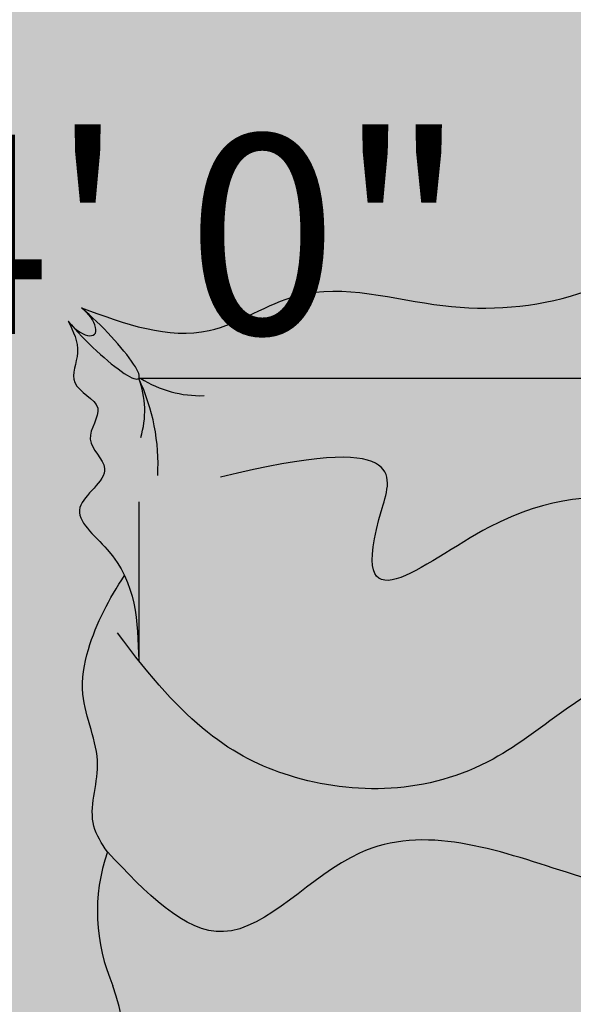
# Model space of a CAD drawing. Units: inches. Extents: x 1704 to 6393, y -157 to 1172.
# Tile 36 of 122: x 2488 to 2526, y 148 to 215. Entities that reach past the tile are written whole.
import ezdxf

# ---------------------------------------------------------------- set-up
doc = ezdxf.new("R2010")
doc.units = ezdxf.units.IN
doc.header["$MEASUREMENT"] = 0
for name, color, linetype, lineweight in [('A-ANNO-DIMS', 7, 'Continuous', 13), ('A-FURN', 8, 'Continuous', 18), ('estofado', 7, 'Continuous', 25)]:
    doc.layers.add(name, color=color, linetype=linetype, lineweight=lineweight)
doc.layers.add('A-FLOR-PATT', color=7, linetype='Continuous', lineweight=13, true_color=0xf2f2f2)
doc.styles.get("Standard").update_dxf_attribs({"font": 'arial.ttf'})
doc.dimstyles.get("Standard").update_dxf_attribs({"dimtxt": 6, "dimasz": 2, "dimexe": 0.18, "dimexo": 0.0625, "dimgap": 0.09, "dimtad": 0, "dimtih": 1, "dimtoh": 1, "dimdec": 1, "dimzin": 0, "dimdsep": 46, "dimlunit": 3, "dimtxsty": 'Standard', "dimblk": 'ARCHTICK', "dimcen": 0.09, "dimadec": 0, "dimazin": 0, "dimtfac": 1, "dimtdec": 1, "dimtofl": 0, "dimtmove": 0, "dimatfit": 3, "dimfxl": 1, "dimtolj": 1, "dimtzin": 0, "dimarcsym": 0})

# ---------------------------------------------------------------- blocks, each defined once
blk = doc.blocks.new('Cama Box Regencia LOLA')
at = {"layer": 'estofado', "ltscale": 0.2}
h = blk.add_hatch(color=256, dxfattribs=at)
h.dxf.hatch_style = 1
h.set_gradient(color1=(240, 232, 219), color2=(213, 190, 154), one_color=1, tint=0.7200000286102295, name='CURVED')
edge = h.paths.add_edge_path()
edge.add_spline(control_points=[(0.343533776195045, -0.8455058148597345), (0.2879313990920309, -0.8167160606696484), (0.2054770794474052, -0.7744470032542381), (0.0954193394759386, -0.7742416952675626), (-0.0885363502328574, -0.7276964167006668), (0.2428192566063672, -0.7672518992321216), (0.345087521536243, -0.8076697826234067), (0.3825206986321063, -0.8228555492498799)], knot_values=[0.0056315103357428, 0.0056315103357428, 0.0056315103357428, 0.0056315103357428, 0.1860138916206105, 0.2660015162584448, 0.3570871810327863, 0.5963901805690979, 0.739731738908988, 0.739731738908988, 0.739731738908988, 0.739731738908988], degree=3, periodic=0)
edge.add_spline(control_points=[(0.3825206986325611, -0.8228555492497662), (0.3974221570828149, -0.8135511441712424), (0.4121061736600496, -0.8037181558521524), (0.4266849906532571, -0.7937075488799225)], knot_values=[1.358237767273279, 1.358237767273279, 1.358237767273279, 1.358237767273279, 1.409915662372559, 1.409915662372559, 1.409915662372559, 1.409915662372559], degree=3, periodic=0)
edge.add_spline(control_points=[(0.4266849905698109, -0.7937075489369932), (0.3998777739682282, -0.7821381809783361), (0.3476761897024971, -0.7634757898491671), (0.2670618099601825, -0.7565375622627358), (0.0835725072796549, -0.7192994417154637), (0.288524529784695, -0.7446405493717521), (0.4247448861246994, -0.7759943071475277), (0.4449816270193879, -0.7810438091316882)], knot_values=[0.1043639306803623, 0.1043639306803623, 0.1043639306803623, 0.1043639306803623, 0.1896363068641149, 0.2696239315019491, 0.3607095962762907, 0.6000125958126024, 0.6446217338078729, 0.6446217338078729, 0.6446217338078729, 0.6446217338078729], degree=3, periodic=0)
edge.add_spline(control_points=[(0.4449816270197289, -0.7810438091316882), (0.5029779388527232, -0.7406836481117695), (0.5966687145296419, -0.6736247633211292), (0.7071737530245628, -0.6656573253703187), (0.7517012483331201, -0.6672238302253392)], knot_values=[1.43159032281798, 1.43159032281798, 1.43159032281798, 1.43159032281798, 1.63814180148235, 1.770695287284994, 1.770695287284994, 1.770695287284994, 1.770695287284994], degree=3, periodic=0)
edge.add_arc((0.7481853615017826, -0.767162003811734), 0.0999999999999888, 58.7920033978138, 87.98512997550938, ccw=False)
edge.add_line((0.8000000000000682, -0.6816328085782289), (0.8000000000000682, -0.154802362840428))
edge.add_line((0.8000000000000682, -0.154802362840428), (-0.7999999999999546, -0.154802362840428))
edge.add_line((-0.7999999999999546, -0.154802362840428), (-0.8000000000000682, -0.7409839258539819))
edge.add_spline(control_points=[(-0.799999999999841, -0.7409839258539251), (-0.7846451382113174, -0.74846387981205), (-0.7568940913494089, -0.7651582159765554), (-0.7559936909002545, -0.8096905380045313), (-0.7049413305308008, -0.8142555457367848), (-0.7013836936888538, -0.8139988647640733)], knot_values=[0.0122267587020837, 0.0122267587020837, 0.0122267587020837, 0.0122267587020837, 0.0594720782072034, 0.1062176618094138, 0.134458043575382, 0.134458043575382, 0.134458043575382, 0.134458043575382], degree=3, periodic=0)
edge.add_spline(control_points=[(-0.7013836936890812, -0.8139988647637892), (-0.6428309483887916, -0.8132695376718857), (-0.532520673001045, -0.8118955240036598), (-0.2390712668254764, -0.6717984706609172), (-0.3892411364554391, -0.7557901092520752), (-0.4591093260188473, -0.8070101468627512), (-0.5571511178645779, -0.795652750469742), (-0.608497950975675, -0.8409486634728295), (-0.6632498050151981, -0.8266781836207997), (-0.6991149398675134, -0.8254126024436914), (-0.719552182989446, -0.8246914287938125)], knot_values=[0, 0, 0, 0, 0.2187005959148062, 0.4120203559900679, 0.4786136596093368, 0.6046444033330721, 0.6969970394608519, 0.7456449795902803, 0.7925683322559657, 0.8547274388453192, 0.8547274388453192, 0.8547274388453192, 0.8547274388453192], degree=3, periodic=0)
edge.add_spline(control_points=[(-0.7195521829781911, -0.824691428792164), (-0.7293124663336812, -0.8248308281530967), (-0.7545977292818407, -0.8216412233076653), (-0.7742556984202338, -0.794819860189591), (-0.7939222919129634, -0.7820064600295497), (-0.799999999999841, -0.7800193173443404)], knot_values=[0.1564883932805935, 0.1564883932805935, 0.1564883932805935, 0.1564883932805935, 0.184397548386913, 0.2313764834161266, 0.2505984550882281, 0.2505984550882281, 0.2505984550882281, 0.2505984550882281], degree=3, periodic=0)
edge.add_line((-0.8000000000000682, -0.7800193173444541), (-0.7999999999999546, -0.8218505664627286))
edge.add_spline(control_points=[(-0.7999999999999546, -0.8218505664625013), (-0.7938082505512511, -0.8290217081292894), (-0.7673857405620766, -0.8512914803976059), (-0.7619109683460011, -0.8661369353891359), (-0.6555700939965164, -0.8510070218793543), (-0.7139793977868294, -0.8637526923380391), (-0.7379026254519659, -0.8623504601624176), (-0.7688129786438367, -0.8813042143888196), (-0.7854260296310259, -0.8561610219318254), (-0.7961930533253962, -0.8566031243811949), (-0.7999999999999546, -0.8573491405791173)], knot_values=[0.0595743221876141, 0.0595743221876141, 0.0595743221876141, 0.0595743221876141, 0.08075289116965, 0.1037414994169835, 0.1697200936249022, 0.1760361327243865, 0.2071371586311508, 0.2404744334261798, 0.2623408547027293, 0.2736604507987723, 0.2736604507987723, 0.2736604507987723, 0.2736604507987723], degree=3, periodic=0)
edge.add_line((-0.7999999999999546, -0.8573491405791173), (-0.8000000000000682, -0.9113562424721521))
edge.add_spline(control_points=[(-0.8000000000000682, -0.9113562424720385), (-0.7937204054647964, -0.9077594990848183), (-0.7710343135782978, -0.8978798065321029), (-0.7213062468074442, -0.9144666877443228), (-0.6268586829058905, -0.862430497409548), (-0.6896594748232019, -0.9045634991654196), (-0.7483442493064559, -0.9189273406958591), (-0.7835301183422417, -0.922920432793262), (-0.7896301351460125, -0.9477657000142585), (-0.7975786973822779, -0.955260590410262), (-0.8000000000001818, -0.9571831923294098)], knot_values=[0.0138560263374175, 0.0138560263374175, 0.0138560263374175, 0.0138560263374175, 0.0348737775836104, 0.0888666909546002, 0.1078792274429341, 0.1267378491223226, 0.1587140219647659, 0.1937574699451985, 0.2174867851300671, 0.2267221218327879, 0.2267221218327879, 0.2267221218327879, 0.2267221218327879], degree=3, periodic=0)
edge.add_line((-0.7999999999999546, -0.957183192329296), (-0.7999999999999546, -1.145824641594742))
edge.add_spline(control_points=[(-0.8000000000002955, -1.145824641594913), (-0.7271039467997298, -1.094596787649038), (-0.4885706936571524, -0.9465888221489535), (-0.0701640902225336, -0.9707493165000187), (0.237911901821235, -0.902164522332157), (0.3435337762145991, -0.845505814843193)], knot_values=[0.1168958193629841, 0.1168958193629841, 0.1168958193629841, 0.1168958193629841, 0.3797203297758731, 0.9577018633805092, 1.31379338443587, 1.31379338443587, 1.31379338443587, 1.31379338443587], degree=3, periodic=0)
h.paths.add_polyline_path([(-0.6766340706021765, -0.6101327540145576, -0.3575266660906883), (-0.7312746368313583, -0.6354535276154252, -0.3575266660894137), (-0.7059538632299791, -0.5808129613865844, -0.1647847126465284), (-0.7059538632300928, -0.2676124402649407, -0.3575266660890756), (-0.7312746368312446, -0.2129718740360431, -0.3575266660908716), (-0.6766340706020629, -0.2382926476369676, -0.0925607043966334), (-0.1295169377724505, -0.2382926476369107, -0.3575266660898965), (-0.0748763715433825, -0.2129718740360431, -0.3575266660894428), (-0.1001971451446479, -0.2676124402649407, -0.1647847126465285), (-0.1001971451445343, -0.5808129613865844, -0.3575266660890756), (-0.0748763715433825, -0.6354535276154821, -0.3575266660898962), (-0.1295169377724505, -0.6101327540146145, -0.0925607043966531)], flags=16)
h.paths.add_polyline_path([(0.0748763715433825, -0.6354535276157094, -0.3575266660910266), (0.1001971451446479, -0.5808129613865844, -0.1647847126465284), (0.1001971451445343, -0.2676124402649407, -0.3575266660890757), (0.0748763715433825, -0.2129718740360431, -0.3575266660898962), (0.1295169377724505, -0.2382926476369107, -0.0925607043966334), (0.6766340706020629, -0.2382926476369676, -0.3575266660908718), (0.7312746368312446, -0.2129718740360431, -0.3575266660894425), (0.7059538632299791, -0.2676124402649407, -0.1647847126465283), (0.7059538632300928, -0.5808129613865844, -0.3575266660890756), (0.7312746368312446, -0.6354535276154821, -0.3575266660908716), (0.6766340706020629, -0.6101327540145576, -0.0925607043966335), (0.1295169377724505, -0.6101327540146145, -0.3575266660906303)], flags=16)
h = blk.add_hatch(color=256, dxfattribs=at)
h.dxf.hatch_style = 1
h.set_gradient(color1=(206, 178, 131), color2=(227, 212, 186), one_color=1, tint=0.8100000023841857, name='CYLINDER')
edge = h.paths.add_edge_path()
edge.add_arc((0.7481853614966667, -0.7671620038115634), 0.0999999999999888, 342.0511336145294, 447.9851299725766)
edge.add_spline(control_points=[(0.7517012483331201, -0.6672238302253392), (0.7071737530245628, -0.6656573253703187), (0.5966687145298692, -0.6736247633211292), (0.5029779388527232, -0.7406836481117125), (0.4449816270195015, -0.7810438091316314)], knot_values=[1.431590322817835, 1.431590322817835, 1.431590322817835, 1.431590322817835, 1.564143808620479, 1.770695287284994, 1.770695287284994, 1.770695287284994, 1.770695287284994], degree=3, periodic=0)
edge.add_spline(control_points=[(0.4449816270195015, -0.7810438091316314), (0.4388957332065502, -0.7852790380018178), (0.4327996148541616, -0.7895089160493285), (0.4266849906533708, -0.7937075488798087)], knot_values=[1.409915662372814, 1.409915662372814, 1.409915662372814, 1.409915662372814, 1.431590322817835, 1.431590322817835, 1.431590322817835, 1.431590322817835], degree=3, periodic=0)
edge.add_spline(control_points=[(0.4266849906533708, -0.7937075488798087), (0.4121061736600496, -0.8037181558521524), (0.3974221570825875, -0.8135511441712991), (0.38252069863222, -0.8228555492498799)], knot_values=[1.358237767273037, 1.358237767273037, 1.358237767273037, 1.358237767273037, 1.409915662372815, 1.409915662372815, 1.409915662372815, 1.409915662372815], degree=3, periodic=0)
edge.add_line((0.3825206986330158, -0.8228555492493114), (0.343533776286904, -0.8455058148063584))
edge.add_spline(control_points=[(0.3435337761924302, -0.8455058148550165), (0.2379119018048641, -0.902164522335795), (-0.0701640902311738, -0.9707493164995071), (-0.4885706936571524, -0.9465888221488967), (-0.7271039467997298, -1.094596787649038), (-0.8000000000000682, -1.145824641594742)], knot_values=[0.1168958193630798, 0.1168958193630798, 0.1168958193630798, 0.1168958193630798, 0.472987340393773, 1.050968873998409, 1.313793384411202, 1.313793384411202, 1.313793384411202, 1.313793384411202], degree=3, periodic=0)
edge.add_spline(control_points=[(-0.8000000000000682, -1.145824641594742), (-0.8038896190357718, -1.14855807951244), (-0.8077744942224853, -1.151305646504738), (-0.8116551946761774, -1.154065647517199)], knot_values=[0.1028719158199011, 0.1028719158199011, 0.1028719158199011, 0.1028719158199011, 0.1168958193630799, 0.1168958193630799, 0.1168958193630799, 0.1168958193630799], degree=3, periodic=0)
edge.add_arc((-0.7536973518524519, -1.235557294053705), 0.1000000000000352, 125.4208969883762, 169.6981795679068)
edge.add_spline(control_points=[(-0.852085287466366, -1.217673946333093), (-0.8521399740518518, -1.217974812833915), (-0.8565649010855622, -1.242328483616745), (-0.8662697220019026, -1.297321141147904), (-0.8487158298532904, -1.34896742172242), (-0.8348745804664758, -1.381844109035796)], knot_values=[0.3128349436863077, 0.3128349436863077, 0.3128349436863077, 0.3128349436863077, 0.3137509534211996, 0.386958004641742, 0.4759027329026081, 0.4759027329026081, 0.4759027329026081, 0.4759027329026081], degree=3, periodic=0)
edge.add_spline(control_points=[(-0.8348745804664758, -1.38184410903591), (-0.8226532004149476, -1.367823298399059), (-0.8056354908857201, -1.352141651537124), (-0.7460155199962628, -1.32170802000337)], knot_values=[0.0062456970656236, 0.0062456970656236, 0.0062456970656236, 0.0062456970656236, 0.0554759259147193, 0.0554759259147193, 0.0554759259147193, 0.0554759259147193], degree=3, periodic=0)
edge.add_spline(control_points=[(-0.7460155200169539, -1.321708019985464), (-0.6188339616464873, -1.25080943574278), (-0.3488365122128698, -1.179158668568902), (0.0338148848931041, -1.279726484458706), (0.3977250465933366, -1.412092721352792), (0.6449024721503065, -1.106270719748692), (0.7873766543807506, -1.256744909425322), (0.8547271521993025, -1.327877176513538)], knot_values=[0.0991852523588446, 0.0991852523588446, 0.0991852523588446, 0.0991852523588446, 0.5236467270390676, 0.9270872950244264, 1.289918234564769, 1.564439021262726, 1.810554634340498, 1.810554634340498, 1.810554634340498, 1.810554634340498], degree=3, periodic=0)
edge.add_arc((0.5509678495186563, -1.223443291813453), 0.3212104454069235, 341.0267878798241, 383.7782184284114)
edge.add_arc((1.292676354991499, -0.9435407756057543), 0.4723459732861395, 162.0511336103901, 198.5657216587827, ccw=False)
h = blk.add_hatch(color=256, dxfattribs=at)
h.dxf.hatch_style = 1
h.set_gradient(color1=(206, 178, 131), color2=(233, 221, 200), one_color=1, tint=0.8500000238418579, name='CURVED')
edge = h.paths.add_edge_path()
edge.add_spline(control_points=[(0.9233883396182136, -2.254908822900802), (0.9143712174658276, -2.237158585978875), (0.8971704820246486, -2.20329887728792), (0.9295105801843419, -2.140290914518345), (0.848651568119294, -2.10957861148239), (0.9047062348403186, -2.046222426005954), (0.8299480774321636, -1.990932361540615), (0.9387479200587449, -1.92692496801726), (0.8590435458045249, -1.86767849203585), (0.8322262745575699, -1.826028043643361), (0.8247981799574972, -1.810442049687992)], knot_values=[0, 0, 0, 0, 0.0575832900035364, 0.1098437972159638, 0.1698138218664432, 0.2255174829302509, 0.2824861515521905, 0.3632291183773252, 0.4509842065695901, 0.5012091817853866, 0.5012091817853866, 0.5012091817853866, 0.5012091817853866], degree=3, periodic=0)
edge.add_spline(control_points=[(0.8247981799572698, -1.810442049688447), (0.8512430237993839, -1.769990096378137), (0.8869160776755506, -1.705010622333873), (0.9070359522544322, -1.586338752195842), (0.8536462472426364, -1.488247672851343), (0.8944567470317679, -1.387739666353695), (0.8643796102055603, -1.342420998864781), (0.8547271521993025, -1.327877176513538)], knot_values=[0, 0, 0, 0, 0.1438744691785906, 0.2224893870322766, 0.3492927143212738, 0.4561786976395368, 0.5066917301592304, 0.5066917301592304, 0.5066917301592304, 0.5066917301592304], degree=3, periodic=0)
edge.add_spline(control_points=[(0.8547271521993025, -1.327877176513538), (0.7873766543807506, -1.256744909425322), (0.6449024721503065, -1.106270719748692), (0.3977250465933366, -1.412092721352792), (0.0338148848931041, -1.279726484458706), (-0.3488365122128698, -1.179158668568902), (-0.6188339616464873, -1.25080943574278), (-0.7460155200169539, -1.321708019985464)], knot_values=[0.0991852523588446, 0.0991852523588446, 0.0991852523588446, 0.0991852523588446, 0.3453008654366167, 0.6198216521345741, 0.9826525916749167, 1.386093159660275, 1.810554634340498, 1.810554634340498, 1.810554634340498, 1.810554634340498], degree=3, periodic=0)
edge.add_spline(control_points=[(-0.7460155199962628, -1.32170802000337), (-0.8056354908857201, -1.352141651537124), (-0.8226532004149476, -1.367823298399059), (-0.8348745804664758, -1.38184410903591)], knot_values=[0.0062456970656236, 0.0062456970656236, 0.0062456970656236, 0.0062456970656236, 0.0554759259147193, 0.0554759259147193, 0.0554759259147193, 0.0554759259147193], degree=3, periodic=0)
edge.add_spline(control_points=[(-0.8348745804664758, -1.38184410903591), (-0.8364250716851984, -1.383622888820184), (-0.8378983647115774, -1.385374937005849), (-0.8393716577378427, -1.387126985191514)], knot_values=[0, 0, 0, 0, 0.0062456970656236, 0.0062456970656236, 0.0062456970656236, 0.0062456970656236], degree=3, periodic=0)
edge.add_arc((-0.6180450437709624, -1.576392779500167), 0.2912164331649039, 139.4648411061637, 203.3711573294546)
edge.add_arc((-0.7011750866292914, -1.609837078845487), 0.2016528082906132, 204.0179006417974, 212.6189639884946)
edge.add_spline(control_points=[(-0.8710220093900034, -1.718537943240505), (-0.8696870122217887, -1.721658691442996), (-0.8597709916446092, -1.746046247230935), (-0.8464685798230674, -1.804421032451443), (-0.888988689927828, -1.889951451602371), (-0.8378676506146121, -1.973422824210047), (-0.8371590179440318, -2.05992368952792), (-0.8871569320951948, -2.144598622072578), (-0.908935644436724, -2.210906123939594), (-0.9233883398977695, -2.254908823284267)], knot_values=[0, 0, 0, 0, 0.0101500649009363, 0.0785829584511912, 0.1732273504791735, 0.2688802694005398, 0.3498050162211252, 0.4202002266429896, 0.5590752189863636, 0.5590752189863636, 0.5590752189863636, 0.5590752189863636], degree=3, periodic=0)
edge.add_ellipse((-0.9040800600764669, -2.258882422916315), major_axis=(0.0267880171833212, 0.0267880171833213), ratio=0.4535320972039226, start_angle=94.15910660291303, end_angle=123.37101895145429, ccw=False)
edge.add_ellipse((-0.8772920428931456, -2.232094405732993), major_axis=(0.0772920428927364, 0.0772920428927364), ratio=0.168252450050839, start_angle=-1.0527401173021644e-10, end_angle=156.3071135567154, ccw=False)
edge.add_line((-0.8000000000002955, -2.154802362840428), (0.7999592378284888, -2.154802362840428))
edge.add_arc((0.9462065466516378, -2.098298447668867), 0.1567831871334379, 200.9447658774159, 201.1244713640487, ccw=False)
edge.add_arc((1.115979327553759, -2.004946707326951), 0.3497136727815615, 205.2898146244752, 205.3730108333857)
edge.add_ellipse((0.8772920428930319, -2.232094405732993), major_axis=(-0.0772920428927364, 0.0772920428927364), ratio=0.168252450050839, start_angle=203.6928864432847, end_angle=359.99999999994674, ccw=False)
edge.add_ellipse((0.9040800600763532, -2.258882422916315), major_axis=(-0.0267880171833213, 0.0267880171833213), ratio=0.4535320972039226, start_angle=236.6289810485458, end_angle=265.84089339708703, ccw=False)
h = blk.add_hatch(color=256, dxfattribs=at)
h.dxf.hatch_style = 1
h.set_gradient(color1=(206, 178, 131), color2=(233, 221, 200), one_color=1, tint=0.8500000238418579, name='CURVED')
edge = h.paths.add_edge_path()
edge.add_spline(control_points=[(-0.9001064604443627, -2.27819070273756), (-0.866259371332262, -2.263084355976445), (-0.8028331991894219, -2.234776522858453), (-0.7685206103102474, -2.343981002846874), (-0.6122536186376238, -2.322828464485212), (-0.4353754265674752, -2.183795504726106), (-0.2043351766035357, -2.412166101990749), (0.035742157155596, -2.28434544697319), (0.2724023732024534, -2.265741378418681), (0.4990197572961961, -2.339647395113615), (0.6925408411253784, -2.202138696866825), (0.8240737498149427, -2.250332331133733), (0.900106460444249, -2.27819070273756)], knot_values=[0, 0, 0, 0, 0.0915194039844232, 0.1714985135733706, 0.2551966802733756, 0.4993431682155844, 0.7776132872898075, 0.9991109890269537, 1.23769004728933, 1.492615491211055, 1.658192352121012, 1.885025012049534, 1.885025012049534, 1.885025012049534, 1.885025012049534], degree=3, periodic=0)
edge.add_ellipse((0.9040800600763532, -2.258882422916315), major_axis=(-0.0267880171833213, 0.0267880171833213), ratio=0.4535320972039226, start_angle=454.1591066084853, end_angle=483.3710189511271, ccw=False)
edge.add_ellipse((0.8772920428930319, -2.232094405732993), major_axis=(-0.0772920428927364, 0.0772920428927364), ratio=0.168252450050839, start_angle=359.99999999994674, end_angle=516.3071135577263, ccw=False)
edge.add_arc((0.9462065466977946, -2.098298447788181), 0.1567831871334379, 201.1244713173118, 201.142614633458, ccw=False)
edge.add_line((0.7999592378286025, -2.154802362840428), (-0.8000000000004092, -2.154802362840428))
edge.add_ellipse((-0.8772920428931456, -2.232094405732993), major_axis=(0.0772920428927364, 0.0772920428927364), ratio=0.168252450050839, start_angle=-156.3071135577261, end_angle=-1.0527401173021644e-10, ccw=False)
edge.add_ellipse((-0.9040800600764669, -2.258882422916315), major_axis=(0.0267880171833212, 0.0267880171833213), ratio=0.4535320972039226, start_angle=-123.3710189511271, end_angle=-94.15910660848522, ccw=False)
h = blk.add_hatch(color=256, dxfattribs=at)
h.dxf.hatch_style = 1
h.set_gradient(color1=(206, 178, 131), color2=(233, 221, 200), one_color=1, tint=0.8500000238418579, name='CURVED')
edge = h.paths.add_edge_path()
edge.add_ellipse((0.8772920428930319, -2.232094405732993), major_axis=(-0.0772920428927364, 0.0772920428927364), ratio=0.168252450050839, start_angle=203.6928864432846, end_angle=359.9999999999468)
edge.add_ellipse((0.8772920428930319, -2.232094405732993), major_axis=(-0.0772920428927364, 0.0772920428927364), ratio=0.168252450050839, start_angle=359.9999999999468, end_angle=516.3071135577261)
edge.add_ellipse((0.9040800600763532, -2.258882422916315), major_axis=(-0.0267880171833213, 0.0267880171833213), ratio=0.4535320972039226, start_angle=265.84089339708703, end_angle=454.1591066084853, ccw=False)
for p, q in [((0.8000000000000682, -1.939064283336335), (0.8000000000000682, -1.662039728679133)), ((-0.7999999999999546, -2.154802362840428), (0.8000000000000682, -2.154802362840428))]:
    blk.add_line(p, q, dxfattribs=at)
for centre, radius, start, end in [((1.292676354991613, -0.9435407756055268), 0.4723459732861117, 162.0511336104213, 198.5657216589983), ((0.55096784951877, -1.223443291813453), 0.3212104454069235, 341.0267878798186, 23.77821842812888), ((1.115979327644367, -2.00494670751874), 0.3497136727815545, 176.7524727679717, 205.3730107986517), ((0.9462065466502735, -2.098298447665399), 0.1567831871334492, 162.6474673821321, 201.1361021892849), ((0.6916068347399005, -2.322769188842187), 0.1980600766927276, 58.0012856468178, 91.6550645032879)]:
    blk.add_arc(centre, radius, start, end, dxfattribs=at)
for centre, major_axis, ratio, start_param, end_param in [((0.8772920428930319, -2.232094405732993), (-0.0772920428927364, 0.0772920428927364), 0.168252450050839, 4.250341947992563, 8.31602866635556), ((0.9040800600763532, -2.258882422916315), (-0.0267880171833213, 0.0267880171833213), 0.4535320972039226, 4.422106649467695, 8.144263964888069)]:
    blk.add_ellipse(centre, major_axis=major_axis, ratio=ratio, start_param=start_param, end_param=end_param, dxfattribs=at)
for points, knots in [([(-0.8116551946761774, -1.154065647517199), (-0.7350455857787211, -1.099579968801037), (-0.493473113061782, -0.9463057365681493), (-0.0701640902311738, -0.9707493164995071), (0.2379119018048641, -0.902164522335795), (0.3435337761924302, -0.8455058148550165)], [0.1028719158199011, 0.1028719158199011, 0.1028719158199011, 0.1028719158199011, 0.3797203297758731, 0.9577018633805092, 1.313793384411202, 1.313793384411202, 1.313793384411202, 1.313793384411202]), ([(-0.7460155200169539, -1.321708019985464), (-0.6188339616464873, -1.25080943574278), (-0.3488365122128698, -1.179158668568902), (0.0338148848931041, -1.279726484458706), (0.3977250465933366, -1.412092721352792), (0.6449024721503065, -1.106270719748692), (0.7873766543807506, -1.256744909425322), (0.8547271521993025, -1.327877176513538)], [0.0991852523588446, 0.0991852523588446, 0.0991852523588446, 0.0991852523588446, 0.5236467270390676, 0.9270872950244264, 1.289918234564769, 1.564439021262726, 1.810554634340498, 1.810554634340498, 1.810554634340498, 1.810554634340498]), ([(0.8547271521993025, -1.327877176513538), (0.8643796102055603, -1.342420998864781), (0.8944567470317679, -1.387739666353695), (0.8536462472426364, -1.488247672851343), (0.9070359522544322, -1.586338752195842), (0.8869160776755506, -1.705010622333873), (0.8512430237993839, -1.769990096378137), (0.8247981799572698, -1.810442049688447)], [0, 0, 0, 0, 0.0505130325196935, 0.1573990158379565, 0.2842023431269537, 0.3628172609806397, 0.5066917301592304, 0.5066917301592304, 0.5066917301592304, 0.5066917301592304]), ([(-0.8337777191962914, -1.686127396833001), (-0.7936227331957753, -1.590003258421234), (-0.5563859991466416, -1.394748990587913), (-0.1321102153461879, -1.783182047565389), (0.1908245506583626, -1.429131816234075), (0.5373208507353411, -1.424480211867205), (0.720102724937533, -1.549855593291283), (0.836774155394778, -1.71068108627179)], [0.0299011711635954, 0.0299011711635954, 0.0299011711635954, 0.0299011711635954, 0.2769669118207226, 0.7971145189980146, 1.093669199334649, 1.464665995707328, 1.788488893467898, 1.788488893467898, 1.788488893467898, 1.788488893467898]), ([(0.9233883396182136, -2.254908822900802), (0.9143712174658222, -2.237158585978864), (0.8971704820247243, -2.203298877287874), (0.9295105801841641, -2.140290914518474), (0.8486515681193482, -2.109578611482328), (0.9047062348404182, -2.046222426005942), (0.8299480774320162, -1.990932361540672), (0.9387479200587655, -1.926924968017257), (0.8039686482702052, -1.826739790434252), (0.8016292922223446, -1.72965583153342), (0.8000000000000682, -1.662039728679133)], [0, 0, 0, 0, 0.0575832900035364, 0.1098437972159638, 0.1698138218664432, 0.2255174829302509, 0.2824861515521905, 0.3632291183773252, 0.4509842065695901, 0.6523445315224259, 0.6523445315224259, 0.6523445315224259, 0.6523445315224259]), ([(-0.6667836004502306, -1.991594303623287), (-0.4801926263546648, -1.924290517138388), (-0.2421721137753821, -1.866692280098163), (0.067250899423243, -2.056782250863193), (0.4752270537671848, -1.673138005031375), (0.3282580065483671, -2.063228784622481), (0.6572625331713198, -1.982435509858419)], [0.0299011711635954, 0.0299011711635954, 0.0299011711635954, 0.0299011711635954, 0.2769669118207226, 0.7971145189980146, 1.093669199334649, 1.16835959978728, 1.16835959978728, 1.16835959978728, 1.16835959978728]), ([(0.900106460444249, -2.27819070273756), (0.8240737498147286, -2.250332331133789), (0.6925408411252015, -2.202138696866918), (0.4990197572963532, -2.33964739511349), (0.2724023732023884, -2.265741378418779), (0.0357421571555867, -2.284345446973105), (-0.204335176603578, -2.412166101990773), (-0.4353754265674596, -2.183795504726199), (-0.6122536186375224, -2.322828464485116), (-0.7685206103102122, -2.343981002846907), (-0.8028331991894692, -2.234776522858419), (-0.8662593713322198, -2.263084355976456), (-0.9001064604443627, -2.27819070273756)], [0, 0, 0, 0, 0.2268326599285221, 0.3924095208384793, 0.6473349647602045, 0.8859140230225809, 1.107411724759727, 1.38568184383395, 1.629828331776159, 1.713526498476164, 1.793505608065111, 1.885025012049534, 1.885025012049534, 1.885025012049534, 1.885025012049534])]:
    blk.add_open_spline(points, degree=3, knots=knots, dxfattribs=at)
blk = doc.blocks.new('_ArchTick')
at = {"color": 0, "linetype": 'ByBlock', "const_width": 0.15}
blk.add_lwpolyline([(-0.5, -0.5), (0.5, 0.5)], dxfattribs=at)
blk = doc.blocks.new('*D93')
at = {"layer": 'A-ANNO-DIMS', "color": 0, "lineweight": -2, "transparency": 16777216}
for p, q in [((2605.286074000001, 895.2129740000005), (1829.697551000002, 895.2129740000003)), ((1829.877551000002, 895.2129740000003), (1829.877551000002, 495.8664119263302)), ((1829.877551000002, 90.2129739999999), (1829.877551000002, 489.5595360736699)), ((2605.286074000001, 90.21297400000003), (1829.697551000002, 90.2129739999999))]:
    blk.add_line(p, q, dxfattribs=at)
at = {"layer": 'Defpoints', "color": 0, "lineweight": -3, "transparency": 16777216}
for p in [(2605.348574000001, 895.2129740000005), (1829.877551000002, 90.2129739999999), (2605.348574000001, 90.21297400000003)]:
    blk.add_point(p, dxfattribs=at)
at = {"layer": 'A-ANNO-DIMS', "color": 0, "lineweight": -2, "transparency": 16777216, "xscale": 2, "yscale": 2, "zscale": 2}
for p, rotation in [((1829.877551000002, 895.2129740000003), 90), ((1829.877551000002, 90.2129739999999), 270)]:
    blk.add_blockref('_ArchTick', p, dxfattribs=dict(at, rotation=rotation))
at = {"layer": 'A-ANNO-DIMS', "color": 0, "transparency": 16777216, "insert": (1829.877551000001, 492.7129739999994), "char_height": 6, "attachment_point": 5}
blk.add_mtext('\\A1;805', dxfattribs=at)
blk = doc.blocks.new('*D105')
at = {"layer": 'A-ANNO-DIMS', "color": 0, "lineweight": -2, "transparency": 16777216}
for p, q in [((2451.737975, 615.150474), (2451.737975, -64.9670259999999)), ((2547.348574, 615.150474), (2547.348574, -64.9670259999999)), ((2451.737975, -64.787026), (2489.908936164393, -64.787026)), ((2547.348574, -64.787026), (2509.177612835607, -64.787026))]:
    blk.add_line(p, q, dxfattribs=at)
at = {"layer": 'Defpoints', "color": 0, "lineweight": -3, "transparency": 16777216}
for p in [(2451.737975, 615.212974), (2547.348574, 615.212974), (2547.348574, -64.787026)]:
    blk.add_point(p, dxfattribs=at)
at = {"layer": 'A-ANNO-DIMS', "color": 0, "lineweight": -2, "transparency": 16777216, "xscale": 2, "yscale": 2, "zscale": 2, "rotation": 180}
blk.add_blockref('_ArchTick', (2451.737975, -64.787026), dxfattribs=at)
at = {"layer": 'A-ANNO-DIMS', "color": 0, "lineweight": -2, "transparency": 16777216, "xscale": 2, "yscale": 2, "zscale": 2}
blk.add_blockref('_ArchTick', (2547.348574, -64.787026), dxfattribs=at)
at = {"layer": 'A-ANNO-DIMS', "color": 0, "transparency": 16777216, "insert": (2499.5432745, -64.787026), "char_height": 6, "attachment_point": 5}
blk.add_mtext('\\A1;95.61', dxfattribs=at)

msp = doc.modelspace()

# ---------------------------------------------------------------- hatches: boundary and pattern name
at = {"layer": 'A-FLOR-PATT', "transparency": 33554528}
h = msp.add_hatch(color=256, dxfattribs=at)
h.dxf.hatch_style = 1
h.paths.add_polyline_path([(2325.348574056059, 863.2129735309796), (2325.348574056059, 887.2129735309796), (2263.348574056059, 887.2129735309796), (2167.348574056059, 887.2129735309794), (2081.348574056061, 887.2129735309792), (2081.348574056061, 719.2129735309785), (2277.348574056059, 719.2129735309787), (2277.348574056059, 711.2129735309788), (2277.348574056059, 372.212973530979), (2349.348574056059, 372.212973530979), (2381.348574056059, 372.2129735309789), (2381.348574056059, 364.2129735309789), (2353.348574056059, 364.2129735309789), (2353.348574056059, 270.2129735309788), (2381.348574056059, 270.2129735309788), (2381.348574056059, 266.2129735309788), (2357.348574056059, 266.2129735309788), (2357.348574056059, 98.21297353097884), (2381.348574056059, 98.21297353097897), (2385.181056550604, 98.21297353097884), (2386.482186711948, 98.21297353097884), (2424.21496140017, 98.21297353097884), (2425.516091561514, 98.21297353097884), (2429.348574056059, 98.21297353097897), (2597.348574056059, 98.21297353097884), (2597.348574056059, 146.2129735309788), (2597.348574056059, 218.2129735309788), (2597.348574056059, 266.2129735309788), (2423.348574056059, 266.2129735309788), (2423.348574056059, 270.2129735309788), (2473.348574056059, 270.2129735309788), (2473.348574056059, 294.2129735309789), (2477.348574056059, 294.2129735309789), (2477.348574056059, 270.2129735309788), (2547.348574056059, 270.2129735309788), (2547.348574056059, 364.2129735309788), (2477.348574056059, 364.2129735309788), (2477.348574056059, 318.2129735309788), (2473.348574056059, 318.2129735309787), (2473.348574056059, 364.2129735309789), (2423.348574056059, 364.2129735309788), (2423.348574056059, 372.2129735309788), (2469.348574056059, 372.2129735309788), (2469.348574056059, 459.2129735309789), (2469.348574056059, 538.2129735309788), (2350.348574056059, 538.2129735309788), (2350.348574056059, 565.7129735309788), (2358.348574056059, 565.7129735309788), (2358.348574056059, 545.2129735309788), (2420.348574056059, 545.2129735309788), (2420.348574056059, 610.2129735309788), (2358.348574056059, 610.2129735309788), (2358.348574056059, 589.7129735309788), (2350.348574056059, 589.7129735309788), (2350.348574056059, 615.2129735309788), (2425.348574056059, 615.2129735309788), (2425.348574056059, 607.2129735309788), (2425.348574056059, 546.2129735309788), (2469.348574056059, 546.2129735309788), (2514.34857405606, 546.212973530979), (2514.34857405606, 607.2129735309788), (2449.348574056059, 607.2129735309788), (2449.348574056059, 615.2129735309788), (2451.737974987759, 615.2129735309788), (2451.737974987759, 659.2129735309788), (2427.737974987759, 659.2129735309788), (2427.737974987759, 665.2129735309788), (2367.737974987758, 665.2129735309788), (2367.737974987758, 667.2129735309788), (2367.737974987758, 711.2129735309788), (2325.348574056059, 711.2129735309788), (2325.348574056059, 719.2129735309785), (2325.348574056059, 755.2129735309787), (2325.348574056059, 763.2129735309788)])
h.paths.add_polyline_path([(2233.85817000392, 822.532660166629, -0.1872470486944155), (2233.85817000392, 809.1396667958562), (2231.697030374885, 808.8044951349628, 0.0848927708004382), (2233.130501812631, 814.4858417746204), (2230.423974436808, 814.4858417746204, -0.1042581087707907), (2228.553363812687, 808.3129425443484), (2217.750790159711, 807.1555239386723, -0.2222222222222219), (2217.750790159711, 824.5168030238124), (2228.553363812687, 823.3593844181363, -0.1042581087707933), (2230.423974436808, 817.1864851878643), (2233.130501812631, 817.1864851878643, 0.08489277080044), (2231.697030374885, 822.8678318275219)], flags=16)
h.paths.add_polyline_path([(2213.621360876743, 833.1974425663823), (2213.621360876743, 798.4748843961024), (2156.047684459484, 798.4748843961034), (2156.047684459485, 833.1974425663813)], flags=16)
h.paths.add_polyline_path([(2203.931929661768, 848.0987249710489), (2205.089348267444, 837.2961513180724, -0.2222222222222264), (2187.728069182304, 837.2961513180724), (2188.88548778798, 848.0987249710485, -0.104258108770792), (2195.058387018252, 849.9693355951691), (2195.058387018252, 852.6758629709927, 0.084892770800438), (2189.377040378595, 851.2423915332469), (2189.712212039488, 853.4035311622828, -0.1872470486944166), (2203.105205410261, 853.4035311622828), (2203.440377071154, 851.2423915332469, 0.084892770800438), (2197.759030431496, 852.6758629709927), (2197.759030431496, 849.9693355951691, -0.1042581087707896)], flags=16)
h.paths.add_polyline_path([(2181.940976153924, 837.2961513180726, -0.2222222222222323), (2164.579697068783, 837.2961513180724), (2165.73711567446, 848.0987249710487, -0.1042581087707905), (2171.910014904732, 849.9693355951691), (2171.910014904732, 852.6758629709927, 0.0848927708004445), (2166.228668265074, 851.2423915332469), (2166.563839925967, 853.403531162283, -0.1872470486944096), (2179.95683329674, 853.4035311622828), (2180.292004957633, 851.2423915332465, 0.0848927708004458), (2174.610658317976, 852.6758629709927), (2174.610658317976, 849.9693355951691, -0.104258108770801), (2180.783557548248, 848.0987249710482)], flags=16)
h.paths.add_polyline_path([(2205.089348267444, 794.376175644412), (2203.931929661768, 783.5736019914364, -0.1042581087707934), (2197.759030431496, 781.7029913673155), (2197.759030431496, 778.9964639914921, 0.084892770800439), (2203.440377071154, 780.4299354292382), (2203.105205410261, 778.2687958002022, -0.1872470486944172), (2189.712212039488, 778.2687958002018), (2189.377040378595, 780.4299354292377, 0.0848927708004369), (2195.058387018252, 778.9964639914919), (2195.058387018252, 781.7029913673153, -0.1042581087707904), (2188.88548778798, 783.5736019914358), (2187.728069182304, 794.3761756444126, -0.2222222222222231)], flags=16)
h.paths.add_polyline_path([(2181.940976153924, 794.376175644412), (2180.783557548248, 783.5736019914364, -0.1042581087708008), (2174.610658317976, 781.7029913673153), (2174.610658317976, 778.9964639914921, 0.0848927708004458), (2180.292004957633, 780.4299354292382), (2179.95683329674, 778.268795800202, -0.1872470486944096), (2166.563839925967, 778.2687958002018), (2166.228668265074, 780.4299354292378, 0.0848927708004446), (2171.910014904732, 778.9964639914919), (2171.910014904732, 781.7029913673153, -0.1042581087707904), (2165.73711567446, 783.5736019914358), (2164.579697068783, 794.3761756444123, -0.2222222222222294)], flags=16)
h.paths.add_polyline_path([(2151.918255176517, 807.1555239386723), (2141.115681523541, 808.3129425443484, -0.1042581087707911), (2139.24507089942, 814.4858417746204), (2136.538543523597, 814.4858417746204, 0.08489277080044), (2137.972014961343, 808.8044951349626), (2135.810875332307, 809.1396667958562, -0.1872470486944109), (2135.810875332307, 822.5326601666285), (2137.972014961343, 822.8678318275221, 0.0848927708004416), (2136.538543523597, 817.1864851878643), (2139.24507089942, 817.1864851878643, -0.104258108770793), (2141.115681523541, 823.3593844181363), (2151.918255176517, 824.5168030238124, -0.2222222222222205)], flags=16)
h.paths.add_polyline_path([(2357.868011454448, 363.4102250290031), (2358.813881560335, 363.4102250290031, 0.7537604849588476)], flags=16)
h.paths.add_polyline_path([(2372.241054283868, 363.1167008961685), (2372.248110816919, 363.1167008961685), (2372.248110816919, 363.3425764997267), (2371.30224071103, 363.3425764997267), (2371.30224071103, 363.1392706554335, -1.360391292333951)], flags=16)
h.paths.add_polyline_path([(2371.309297244092, 272.7157694655011), (2371.30224071103, 272.7157694655011), (2371.30224071103, 272.4898938619428), (2372.248110816919, 272.4898938619428), (2372.248110816919, 272.6931997062759, -1.360391292393621)], flags=16)
h.paths.add_polyline_path([(2357.875067987504, 272.7157694655011), (2357.868011454452, 272.7157694655011), (2357.868011454452, 272.4898938619428), (2358.813881560341, 272.4898938619428), (2358.813881560341, 272.6931997062361, -1.360391292333948)], flags=16)
h.paths.add_polyline_path([(2353.768696905258, 363.0736921025416), (2376.347425366111, 363.0736921025416), (2376.347425366111, 272.7587782591281), (2353.768696905258, 272.7587782591281)], flags=16)
h.paths.add_polyline_path([(2354.772195947961, 362.0701930598379), (2375.343926323407, 362.0701930598379), (2375.343926323407, 273.7622773018316), (2354.772195947961, 273.7622773018318)], flags=0)
h.paths.add_polyline_path([(2357.868011454452, 363.3425764997267), (2358.813881560341, 363.3425764997266), (2358.813881560341, 363.1167008961684), (2357.868011454452, 363.1167008961684)], flags=16)
h.paths.add_polyline_path([(2359.287941640134, 359.1843485433627), (2359.287941640134, 360.0631949744305), (2370.828180631237, 360.0631949744362), (2370.828180631237, 359.1843485433769), (2374.332057422314, 359.1843485433812), (2374.332057422312, 358.4635369582513), (2372.835178716611, 358.4635369582524), (2372.835178716611, 357.5410357047662), (2374.332057422314, 357.5410357047678), (2374.332057422312, 356.8202241196381), (2372.835178716611, 356.820224119639), (2372.835178716611, 355.897722866153), (2374.332057422314, 355.8977228661546), (2374.332057422312, 355.1769112810248), (2372.835178716611, 355.1769112810259), (2372.835178716611, 354.2544100275397), (2374.332057422334, 354.2544100275415), (2374.332057422331, 353.5335984424117), (2372.835178716631, 353.5335984424126), (2372.835178716631, 352.6110971889265), (2374.332057422334, 352.6110971889282), (2374.332057422331, 351.8902856037984), (2372.835178716631, 351.8902856037993), (2372.835178716631, 350.9677843503132), (2374.332057422334, 350.967784350315), (2374.332057422331, 350.2469727651852), (2372.835178716631, 350.2469727651861), (2372.835178716631, 349.3244715117), (2374.332057422334, 349.3244715117017), (2374.332057422331, 348.603659926572), (2372.835178716631, 348.6036599265729), (2372.835178716631, 347.6811586730868), (2374.332057422334, 347.6811586730886), (2374.332057422331, 346.9603470879587), (2372.835178716631, 346.9603470879598), (2372.835178716631, 346.0378458344735), (2374.332057422334, 346.0378458344753), (2374.332057422331, 345.3170342493456), (2372.835178716631, 345.3170342493465), (2372.835178716631, 344.3945329958605), (2374.332057422334, 344.3945329958621), (2374.332057422331, 343.6737214107324), (2372.835178716631, 343.6737214107334), (2372.835178716631, 342.751220157247), (2374.332057422334, 342.7512201572489), (2374.332057422331, 342.0304085721191), (2372.835178716631, 342.03040857212), (2372.835178716631, 341.1079073186338), (2374.332057422334, 341.1079073186356), (2374.332057422331, 340.3870957335057), (2372.835178716631, 340.3870957335066), (2372.835178716631, 339.4645944800207), (2374.332057422334, 339.4645944800223), (2374.332057422331, 338.7437828948924), (2372.835178716648, 338.7437828948933), (2372.835178716648, 337.8212816414076), (2374.332057422334, 337.8212816414093), (2374.332057422331, 337.1004700562794), (2372.835178716648, 337.1004700562803), (2372.835178716648, 336.1779688027942), (2374.332057422334, 336.1779688027961), (2374.332057422331, 335.4571572176662), (2372.835178716648, 335.4571572176673), (2372.835178716648, 334.5346559641809), (2374.332057422334, 334.5346559641828), (2374.332057422331, 333.8138443790529), (2372.835178716648, 333.8138443790539), (2372.835178716648, 332.8913431255679), (2374.332057422334, 332.8913431255696), (2374.332057422331, 332.1705315404397), (2372.835178716648, 332.1705315404406), (2372.835178716648, 331.2480302869545), (2374.332057422334, 331.2480302869563), (2374.332057422331, 330.5272187018265), (2372.835178716648, 330.5272187018273), (2372.835178716648, 329.6047174483413), (2374.332057422334, 329.6047174483431), (2374.332057422331, 328.8839058632133), (2372.835178716648, 328.8839058632143), (2372.835178716648, 327.9614046097282), (2374.332057422334, 327.9614046097298), (2374.332057422331, 327.2405930246), (2372.835178716648, 327.2405930246009), (2372.835178716648, 326.3180917711149), (2374.332057422334, 326.3180917711167), (2374.332057422331, 325.5972801859869), (2372.835178716648, 325.5972801859877), (2372.835178716648, 324.6747789325016), (2374.332057422334, 324.6747789325034), (2374.332057422331, 323.9539673473736), (2372.835178716648, 323.9539673473746), (2372.835178716648, 323.0314660938884), (2374.332057422334, 323.0314660938901), (2374.332057422331, 322.3106545087603), (2372.835178716648, 322.3106545087613), (2372.835178716648, 321.3881532552753), (2374.332057422334, 321.388153255277), (2374.332057422331, 320.6673416701471), (2372.835178716648, 320.6673416701481), (2372.835178716648, 319.7448404166621), (2374.332057422334, 319.7448404166638), (2374.332057422331, 319.0240288315339), (2372.835178716648, 319.0240288315348), (2372.835178716648, 318.1015275780487), (2374.332057422334, 318.1015275780504), (2374.332057422331, 317.3807159929205), (2372.835178716648, 317.3807159929214), (2372.835178716648, 316.4582147394357), (2374.332057422334, 316.4582147394373), (2374.332057422331, 315.7374031543073), (2372.835178716648, 315.7374031543084), (2372.835178716648, 314.8149019008223), (2374.332057422334, 314.8149019008241), (2374.332057422331, 314.0940903156943), (2372.835178716648, 314.0940903156952), (2372.835178716648, 313.171589062209), (2374.332057422334, 313.1715890622108), (2374.332057422331, 312.450777477081), (2372.835178716648, 312.4507774770819), (2372.835178716648, 311.5282762235959), (2374.332057422334, 311.5282762235977), (2374.332057422331, 310.8074646384678), (2372.835178716648, 310.8074646384687), (2372.835178716648, 309.8849633849827), (2374.332057422334, 309.8849633849844), (2374.332057422331, 309.1641517998546), (2372.835178716648, 309.1641517998555), (2372.835178716648, 308.2416505463693), (2374.332057422334, 308.2416505463712), (2374.332057422331, 307.5208389612412), (2372.835178716648, 307.5208389612421), (2372.835178716648, 306.5983377077562), (2374.332057422334, 306.598337707758), (2374.332057422331, 305.8775261226281), (2372.835178716648, 305.8775261226289), (2372.835178716648, 304.955024869143), (2374.332057422334, 304.9550248691447), (2374.332057422331, 304.2342132840149), (2372.835178716648, 304.2342132840158), (2372.835178716648, 303.3117120305298), (2374.332057422334, 303.3117120305316), (2374.332057422331, 302.5909004454018), (2372.835178716648, 302.5909004454027), (2372.835178716648, 301.6683991919165), (2374.332057422334, 301.6683991919183), (2374.332057422331, 300.9475876067885), (2372.835178716648, 300.9475876067894), (2372.835178716648, 300.0250863533033), (2374.332057422334, 300.025086353305), (2374.332057422331, 299.3042747681752), (2372.835178716648, 299.3042747681761), (2372.835178716648, 298.3817735146902), (2374.332057422334, 298.3817735146919), (2374.332057422331, 297.6609619295621), (2372.835178716648, 297.6609619295629), (2372.835178716648, 296.7384606760769), (2374.332057422334, 296.7384606760786), (2374.332057422331, 296.0176490909488), (2372.835178716648, 296.0176490909498), (2372.835178716648, 295.0951478374636), (2374.332057422334, 295.0951478374653), (2374.332057422331, 294.3743362523355), (2372.835178716648, 294.3743362523364), (2372.835178716648, 293.4518349988504), (2374.332057422334, 293.4518349988522), (2374.332057422331, 292.7310234137224), (2372.835178716648, 292.7310234137233), (2372.835178716648, 291.8085221602371), (2374.332057422334, 291.8085221602389), (2374.332057422331, 291.0877105751091), (2372.835178716648, 291.08771057511), (2372.835178716648, 290.165209321624), (2374.332057422334, 290.1652093216256), (2374.332057422331, 289.4443977364957), (2372.835178716648, 289.4443977364966), (2372.835178716648, 288.5218964830108), (2374.332057422334, 288.5218964830125), (2374.332057422331, 287.8010848978827), (2372.835178716648, 287.8010848978836), (2372.835178716648, 286.8785836443975), (2374.332057422334, 286.8785836443993), (2374.332057422331, 286.1577720592695), (2372.835178716648, 286.1577720592703), (2372.835178716648, 285.2352708057842), (2374.332057422334, 285.2352708057861), (2374.332057422331, 284.5144592206562), (2372.835178716648, 284.514459220657), (2372.835178716648, 283.5919579671712), (2374.332057422334, 283.5919579671728), (2374.332057422331, 282.871146382043), (2372.835178716648, 282.8711463820439), (2372.835178716648, 281.9486451285579), (2374.332057422334, 281.9486451285596), (2374.332057422331, 281.2278335434298), (2372.835178716648, 281.2278335434307), (2372.835178716648, 280.3053322899446), (2374.332057422334, 280.3053322899464), (2374.332057422331, 279.5845207048164), (2372.835178716648, 279.5845207048174), (2372.835178716648, 278.6620194513314), (2374.332057422334, 278.6620194513331), (2374.332057422331, 277.9412078662033), (2372.835178716648, 277.9412078662043), (2372.835178716648, 277.0187066127184), (2374.332057422334, 277.0187066127201), (2374.332057422331, 276.29789502759), (2370.828180631244, 276.2978950275922), (2370.828180631244, 275.7692753872335), (2359.287941640128, 275.7692753872392), (2359.287941640128, 276.2978950275993), (2355.784064849037, 276.2978950276015), (2355.784064849037, 277.0187066126971), (2357.280943554723, 277.0187066126989), (2357.280943554723, 277.9412078662137), (2355.784064849037, 277.9412078662145), (2355.784064849037, 278.6620194513103), (2357.280943554723, 278.6620194513122), (2357.280943554723, 279.5845207048271), (2355.784064849037, 279.584520704828), (2355.784064849037, 280.3053322899236), (2357.280943554723, 280.3053322899253), (2357.280943554723, 281.2278335434403), (2355.784064849037, 281.2278335434412), (2355.784064849037, 281.9486451285369), (2357.280943554723, 281.9486451285387), (2357.280943554723, 282.8711463820535), (2355.784064849037, 282.8711463820543), (2355.784064849037, 283.5919579671501), (2357.280943554723, 283.591957967152), (2357.280943554723, 284.5144592206668), (2355.784064849037, 284.5144592206676), (2355.784064849037, 285.2352708057632), (2357.280943554723, 285.2352708057651), (2357.280943554723, 286.1577720592801), (2355.784064849037, 286.1577720592809), (2355.784064849037, 286.8785836443766), (2357.280943554723, 286.8785836443784), (2357.280943554723, 287.8010848978931), (2355.784064849037, 287.8010848978941), (2355.784064849037, 288.5218964829895), (2357.280943554723, 288.5218964829913), (2357.280943554723, 289.4443977365064), (2355.784064849037, 289.4443977365072), (2355.784064849037, 290.1652093216029), (2357.280943554723, 290.1652093216047), (2357.280943554723, 291.0877105751197), (2355.784064849037, 291.0877105751206), (2355.784064849037, 291.8085221602161), (2357.280943554723, 291.8085221602179), (2357.280943554723, 292.7310234137328), (2355.784064849037, 292.7310234137337), (2355.784064849037, 293.4518349988293), (2357.280943554723, 293.451834998831), (2357.280943554723, 294.3743362523461), (2355.784064849037, 294.3743362523469), (2355.784064849037, 295.0951478374426), (2357.280943554723, 295.0951478374445), (2357.280943554723, 296.0176490909594), (2355.784064849037, 296.0176490909601), (2355.784064849037, 296.7384606760557), (2357.280943554723, 296.7384606760575), (2357.280943554723, 297.6609619295724), (2355.784064849037, 297.6609619295734), (2355.784064849037, 298.3817735146691), (2357.280943554723, 298.3817735146709), (2357.280943554723, 299.3042747681858), (2355.784064849037, 299.3042747681866), (2355.784064849037, 300.0250863532823), (2357.280943554723, 300.0250863532841), (2357.280943554723, 300.9475876067989), (2355.784064849037, 300.9475876067997), (2355.784064849037, 301.6683991918954), (2357.280943554723, 301.6683991918973), (2357.280943554723, 302.5909004454123), (2355.784064849037, 302.5909004454133), (2355.784064849037, 303.3117120305088), (2357.280943554723, 303.3117120305105), (2357.280943554723, 304.2342132840254), (2355.784064849037, 304.2342132840262), (2355.784064849037, 304.9550248691219), (2357.280943554723, 304.9550248691238), (2357.280943554723, 305.8775261226386), (2355.784064849037, 305.8775261226394), (2355.784064849037, 306.5983377077352), (2357.280943554723, 306.5983377077369), (2357.280943554723, 307.5208389612518), (2355.784064849037, 307.5208389612528), (2355.784064849037, 308.2416505463484), (2357.280943554723, 308.2416505463501), (2357.280943554723, 309.1641517998652), (2355.784064849037, 309.1641517998661), (2355.784064849037, 309.8849633849617), (2357.280943554723, 309.8849633849634), (2357.280943554723, 310.8074646384782), (2355.784064849037, 310.8074646384791), (2355.784064849037, 311.5282762235748), (2357.280943554723, 311.5282762235767), (2357.280943554723, 312.4507774770916), (2355.784064849037, 312.4507774770925), (2355.784064849037, 313.171589062188), (2357.280943554723, 313.1715890621898), (2357.280943554723, 314.0940903157049), (2355.784064849037, 314.0940903157058), (2355.784064849037, 314.8149019008013), (2357.280943554723, 314.8149019008032), (2357.280943554723, 315.7374031543179), (2355.784064849037, 315.7374031543187), (2355.784064849037, 316.4582147394146), (2357.280943554723, 316.4582147394165), (2357.280943554723, 317.3807159929311), (2355.784064849037, 317.3807159929321), (2355.784064849037, 318.1015275780277), (2357.280943554723, 318.1015275780295), (2357.280943554723, 319.0240288315445), (2355.784064849037, 319.0240288315454), (2355.784064849037, 319.744840416641), (2357.280943554723, 319.7448404166428), (2357.280943554723, 320.6673416701576), (2355.784064849037, 320.6673416701585), (2355.784064849037, 321.3881532552541), (2357.280943554723, 321.388153255256), (2357.280943554723, 322.3106545087708), (2355.784064849037, 322.3106545087718), (2355.784064849037, 323.0314660938674), (2357.280943554723, 323.0314660938692), (2357.280943554723, 323.9539673473843), (2355.784064849037, 323.9539673473851), (2355.784064849037, 324.6747789324806), (2357.280943554723, 324.6747789324824), (2357.280943554723, 325.5972801859974), (2355.784064849037, 325.5972801859983), (2355.784064849037, 326.3180917710939), (2357.280943554723, 326.3180917710958), (2357.280943554723, 327.2405930246105), (2355.784064849037, 327.2405930246113), (2355.784064849037, 327.9614046097071), (2357.280943554723, 327.961404609709), (2357.280943554723, 328.8839058632238), (2355.784064849037, 328.8839058632245), (2355.784064849037, 329.6047174483202), (2357.280943554723, 329.604717448322), (2357.280943554723, 330.527218701837), (2355.784064849037, 330.5272187018379), (2355.784064849037, 331.2480302869335), (2357.280943554723, 331.2480302869353), (2357.280943554723, 332.1705315404502), (2355.784064849037, 332.170531540451), (2355.784064849037, 332.8913431255468), (2357.280943554723, 332.8913431255486), (2357.280943554723, 333.8138443790634), (2355.784064849037, 333.8138443790642), (2355.784064849037, 334.5346559641599), (2357.280943554723, 334.5346559641618), (2357.280943554723, 335.4571572176767), (2355.784064849037, 335.4571572176776), (2355.784064849037, 336.1779688027732), (2357.280943554723, 336.177968802775), (2357.280943554723, 337.1004700562898), (2355.784064849037, 337.1004700562908), (2355.784064849037, 337.8212816413864), (2357.280943554723, 337.8212816413883), (2357.280943554723, 338.7437828949031), (2355.784064849037, 338.743782894904), (2355.784064849037, 339.4645944799996), (2357.280943554706, 339.4645944800013), (2357.280943554706, 340.3870957335163), (2355.784064849037, 340.3870957335173), (2355.784064849037, 341.1079073186129), (2357.280943554706, 341.1079073186146), (2357.280943554706, 342.0304085721296), (2355.784064849037, 342.0304085721304), (2355.784064849037, 342.7512201572262), (2357.280943554706, 342.751220157228), (2357.280943554706, 343.6737214107429), (2355.784064849037, 343.6737214107437), (2355.784064849037, 344.3945329958394), (2357.280943554706, 344.3945329958412), (2357.280943554706, 345.317034249356), (2355.784064849037, 345.3170342493569), (2355.784064849037, 346.0378458344526), (2357.280943554706, 346.0378458344544), (2357.280943554706, 346.9603470879692), (2355.784064849037, 346.9603470879701), (2355.784064849037, 347.6811586730658), (2357.280943554706, 347.6811586730677), (2357.280943554706, 348.6036599265824), (2355.784064849037, 348.6036599265833), (2355.784064849037, 349.324471511679), (2357.280943554706, 349.3244715116809), (2357.280943554706, 350.2469727651956), (2355.784064849037, 350.2469727651966), (2355.784064849037, 350.9677843502922), (2357.280943554706, 350.9677843502939), (2357.280943554706, 351.8902856038089), (2355.784064849037, 351.8902856038098), (2355.784064849037, 352.6110971889055), (2357.280943554706, 352.6110971889072), (2357.280943554706, 353.5335984424222), (2355.784064849037, 353.533598442423), (2355.784064849037, 354.2544100275187), (2357.280943554686, 354.2544100275204), (2357.280943554686, 355.1769112810354), (2355.784064849017, 355.1769112810362), (2355.784064849017, 355.897722866132), (2357.280943554686, 355.8977228661338), (2357.280943554686, 356.8202241196486), (2355.784064849017, 356.8202241196495), (2355.784064849017, 357.5410357047453), (2357.280943554686, 357.5410357047471), (2357.280943554686, 358.4635369582618), (2355.784064849017, 358.4635369582626), (2355.784064849017, 359.1843485433584)], flags=0)

# ---------------------------------------------------------------- block references
at = {"layer": 'A-FURN', "xscale": 39.22313671019584, "yscale": 39.22313671019584, "zscale": 39.22313671019584, "rotation": 180}
msp.add_blockref('Cama Box Regencia LOLA', (2527.569415053021, 106.0625493409584), dxfattribs=at)

# ---------------------------------------------------------------- texts
at = {"layer": 'A-ANNO-DIMS'}
msp.add_text('20\' 0" X 14\' 0"', height=13.66720297459778, dxfattribs=at).set_placement((2401.140933752799, 193.6187147507726))

# ---------------------------------------------------------------- dimensions: what is measured, and where the dimension line sits
dim = msp.add_linear_dim(base=(1829.877551000002, 90.2129739999999), p1=(2605.348574000001, 895.212974), p2=(2605.348574000001, 90.21297399999999), angle=90, dimstyle='Standard', override={"dimdec": 0, "dimlfac": 1, "dimrnd": 0, "dimzin": 0, "dimdsep": 46, "dimlunit": 2}, dxfattribs=at)
dim.commit()
dim.dimension.update_dxf_attribs({"geometry": '*D93', "text_midpoint": (1829.877551000001, 492.7129739999994)})
dim = msp.add_linear_dim(base=(2547.348574, -64.787026), p1=(2451.737975, 615.212974), p2=(2547.348574, 615.212974), dimstyle='Standard', override={"dimdec": 2, "dimlfac": 1, "dimrnd": 0, "dimzin": 0, "dimdsep": 46, "dimlunit": 2}, dxfattribs=at)
dim.commit()
dim.dimension.update_dxf_attribs({"geometry": '*D105', "text_midpoint": (2499.5432745, -64.787026)})

doc.saveas('drawing.dxf')
